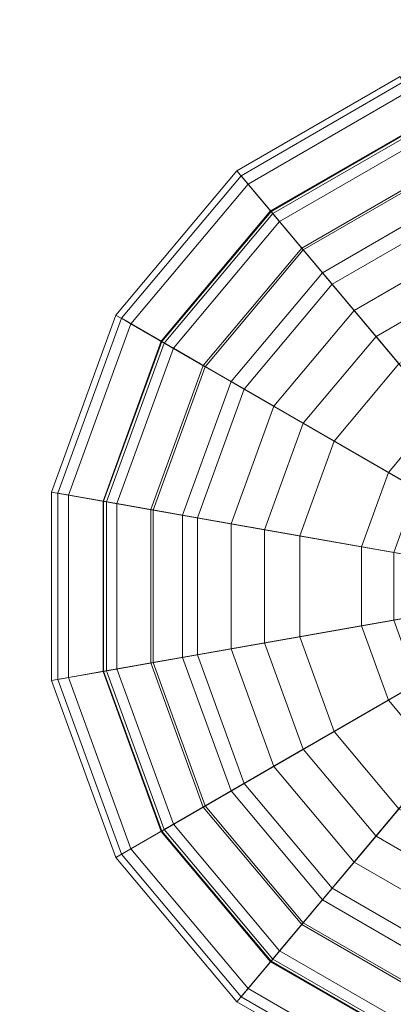
# Model space of a CAD drawing. Units: inches. Extents: x 375 to 1122, y 27 to 1069.
# Tile 128 of 155: x 720.668 to 721.601, y 901.45 to 903.908. Entities that reach past the tile are written whole.
import ezdxf

# ---------------------------------------------------------------- set-up
doc = ezdxf.new("R2010")
doc.units = ezdxf.units.IN
doc.layers.add('A-ANNO-DIMS', color=2, linetype='Continuous', lineweight=18)
doc.layers.add('Furniture', color=30, linetype='Continuous', lineweight=18)
doc.styles.get("Standard").update_dxf_attribs({"font": 'arial.ttf'})
doc.dimstyles.new('ISO-25', dxfattribs={"dimtxt": 12, "dimasz": 2.5, "dimexe": 1.5, "dimexo": 1.5, "dimtad": 1, "dimdec": 1, "dimlunit": 3, "dimtxsty": 'Standard', "dimblk": 'ARCHTICK', "dimcen": 2.5, "dimadec": 0, "dimazin": 0, "dimtfac": 1, "dimtdec": 1, "dimtmove": 0, "dimatfit": 3, "dimfxl": 1.5, "dimfxlon": 1, "dimarcsym": 0})

# ---------------------------------------------------------------- blocks, each defined once
blk = doc.blocks.new('A$C403C54AD')
for points in [[(0.863915, 0.916753, -0.042784), (0.895735, 0.928335, -0.039705), (0.895735, 0.928335, -0.039705), (0.869795, 0.906568, -0.042784)], [(0.869795, 0.906568, -0.042784), (0.895735, 0.928335, -0.039705), (0.895735, 0.928335, -0.039705), (0.878804, 0.899009, -0.042784)], [(0.878804, 0.899009, -0.042784), (0.895735, 0.928335, -0.039705), (0.895735, 0.928335, -0.039705), (0.889855, 0.894987, -0.042784)], [(0.889855, 0.894987, -0.042784), (0.895735, 0.928335, -0.039705), (0.895735, 0.928335, -0.039705), (0.901615, 0.894987, -0.042784)], [(0.921675, 0.906568, -0.042784), (0.895735, 0.928335, -0.039705), (0.895735, 0.928335, -0.039705), (0.927555, 0.916753, -0.042784)], [(0.912666, 0.899009, -0.042784), (0.895735, 0.928335, -0.039705), (0.895735, 0.928335, -0.039705), (0.921675, 0.906568, -0.042784)], [(0.901615, 0.894987, -0.042784), (0.895735, 0.928335, -0.039705), (0.895735, 0.928335, -0.039705), (0.912666, 0.899009, -0.042784)], [(0.876605, 0.921372, 0.050493), (0.886226, 0.924874, 0.043125), (0.887983, 0.92183, 0.043125), (0.88014, 0.915249, 0.050493)], [(0.911329, 0.915249, 0.050493), (0.903486, 0.92183, 0.043125), (0.905243, 0.924874, 0.043125), (0.914864, 0.921372, 0.050493)], [(0.882378, 0.923473, -0.036278), (0.866983, 0.91787, -0.039553), (0.872296, 0.908668, -0.039553), (0.884846, 0.919198, -0.036278)], [(0.906623, 0.919198, -0.036278), (0.919173, 0.908668, -0.039553), (0.924486, 0.91787, -0.039553), (0.909092, 0.923473, -0.036278)], [(0.878701, 0.922135, 0.05268), (0.872606, 0.919916, 0.062072), (0.87688, 0.912514, 0.062072), (0.881848, 0.916683, 0.05268)], [(0.888914, 0.922611, 0.046044), (0.881848, 0.916683, 0.05268), (0.886671, 0.912636, 0.05268), (0.891283, 0.920623, 0.046044)], [(0.900187, 0.920623, 0.046044), (0.904798, 0.912636, 0.05268), (0.909621, 0.916683, 0.05268), (0.902556, 0.922611, 0.046044)], [(0.909621, 0.916683, 0.05268), (0.914589, 0.912514, 0.062072), (0.918863, 0.919916, 0.062072), (0.912769, 0.922135, 0.05268)], [(0.88014, 0.915249, 0.050493), (0.887983, 0.92183, 0.043125), (0.890675, 0.919571, 0.043125), (0.885556, 0.910704, 0.050493)], [(0.905913, 0.910704, 0.050493), (0.900794, 0.919571, 0.043125), (0.903486, 0.92183, 0.043125), (0.911329, 0.915249, 0.050493)], [(0.869965, 0.918955, 0.060725), (0.876605, 0.921372, 0.050493), (0.88014, 0.915249, 0.050493), (0.874727, 0.910707, 0.060725)], [(0.916743, 0.910707, 0.060725), (0.911329, 0.915249, 0.050493), (0.914864, 0.921372, 0.050493), (0.921505, 0.918955, 0.060725)], [(0.869828, 0.918905, 0.119395), (0.874609, 0.920646, 0.129606), (0.878513, 0.913884, 0.129606), (0.874615, 0.910614, 0.119395)], [(0.874609, 0.920646, 0.129606), (0.871716, 0.919593, 0.129606), (0.876155, 0.911905, 0.129606), (0.878513, 0.913884, 0.129606)], [(0.886415, 0.920514, -0.033413), (0.884846, 0.919198, -0.036278), (0.888627, 0.916025, -0.036278), (0.889651, 0.917798, -0.033413)], [(0.891283, 0.920623, 0.046044), (0.886671, 0.912636, 0.05268), (0.892587, 0.910483, 0.05268), (0.894188, 0.919566, 0.046044)], [(0.897281, 0.919566, 0.046044), (0.898882, 0.910483, 0.05268), (0.904798, 0.912636, 0.05268), (0.900187, 0.920623, 0.046044)], [(0.901818, 0.917798, -0.033413), (0.902842, 0.916025, -0.036278), (0.906623, 0.919198, -0.036278), (0.905055, 0.920514, -0.033413)], [(0.912956, 0.913884, 0.129606), (0.915314, 0.911905, 0.129606), (0.919753, 0.919593, 0.129606), (0.91686, 0.920646, 0.129606)], [(0.916854, 0.910614, 0.119395), (0.912956, 0.913884, 0.129606), (0.91686, 0.920646, 0.129606), (0.921641, 0.918905, 0.119395)], [(0.872606, 0.919916, 0.062072), (0.867806, 0.918169, 0.079219), (0.872967, 0.90923, 0.079219), (0.87688, 0.912514, 0.062072)], [(0.914589, 0.912514, 0.062072), (0.918502, 0.90923, 0.079219), (0.923663, 0.918169, 0.079219), (0.918863, 0.919916, 0.062072)], [(0.871716, 0.919593, 0.129606), (0.867021, 0.917884, 0.1202), (0.872327, 0.908694, 0.1202), (0.876155, 0.911905, 0.129606)], [(0.884846, 0.919198, -0.036278), (0.872296, 0.908668, -0.039553), (0.880436, 0.901837, -0.039553), (0.888627, 0.916025, -0.036278)], [(0.885556, 0.910704, 0.050493), (0.890675, 0.919571, 0.043125), (0.893978, 0.91837, 0.043125), (0.8922, 0.908286, 0.050493)], [(0.894188, 0.919566, 0.046044), (0.892587, 0.910483, 0.05268), (0.898882, 0.910483, 0.05268), (0.897281, 0.919566, 0.046044)], [(0.89927, 0.908286, 0.050493), (0.897492, 0.91837, 0.043125), (0.900794, 0.919571, 0.043125), (0.905913, 0.910704, 0.050493)], [(0.902842, 0.916025, -0.036278), (0.911033, 0.901837, -0.039553), (0.919173, 0.908668, -0.039553), (0.906623, 0.919198, -0.036278)], [(0.915314, 0.911905, 0.129606), (0.919142, 0.908694, 0.1202), (0.924448, 0.917884, 0.1202), (0.919753, 0.919593, 0.129606)], [(0.864924, 0.91712, 0.078734), (0.869965, 0.918955, 0.060725), (0.874727, 0.910707, 0.060725), (0.870617, 0.907259, 0.078734)], [(0.867188, 0.917944, 0.106759), (0.869828, 0.918905, 0.119395), (0.874615, 0.910614, 0.119395), (0.872463, 0.908807, 0.106759)], [(0.920852, 0.907259, 0.078734), (0.916743, 0.910707, 0.060725), (0.921505, 0.918955, 0.060725), (0.926546, 0.91712, 0.078734)], [(0.919006, 0.908807, 0.106759), (0.916854, 0.910614, 0.119395), (0.921641, 0.918905, 0.119395), (0.924281, 0.917944, 0.106759)], [(0.866983, 0.91787, -0.039553), (0.863915, 0.916753, -0.042784), (0.869795, 0.906568, -0.042784), (0.872296, 0.908668, -0.039553)], [(0.867021, 0.917884, 0.1202), (0.864289, 0.916889, 0.106976), (0.8701, 0.906825, 0.106976), (0.872327, 0.908694, 0.1202)], [(0.867806, 0.918169, 0.079219), (0.867188, 0.917944, 0.106759), (0.872463, 0.908807, 0.106759), (0.872967, 0.90923, 0.079219)], [(0.8922, 0.908286, 0.050493), (0.893978, 0.91837, 0.043125), (0.897492, 0.91837, 0.043125), (0.89927, 0.908286, 0.050493)], [(0.918502, 0.90923, 0.079219), (0.919006, 0.908807, 0.106759), (0.924281, 0.917944, 0.106759), (0.923663, 0.918169, 0.079219)], [(0.919142, 0.908694, 0.1202), (0.921369, 0.906825, 0.106976), (0.92718, 0.916889, 0.106976), (0.924448, 0.917884, 0.1202)], [(0.919173, 0.908668, -0.039553), (0.921675, 0.906568, -0.042784), (0.927555, 0.916753, -0.042784), (0.924486, 0.91787, -0.039553)], [(0.889651, 0.917798, -0.033413), (0.888627, 0.916025, -0.036278), (0.893266, 0.914336, -0.036278), (0.893622, 0.916353, -0.033413)], [(0.897847, 0.916353, -0.033413), (0.898203, 0.914336, -0.036278), (0.902842, 0.916025, -0.036278), (0.901818, 0.917798, -0.033413)], [(0.864289, 0.916889, 0.106976), (0.864924, 0.91712, 0.078734), (0.870617, 0.907259, 0.078734), (0.8701, 0.906825, 0.106976)], [(0.881848, 0.916683, 0.05268), (0.87688, 0.912514, 0.062072), (0.883428, 0.907019, 0.062072), (0.886671, 0.912636, 0.05268)], [(0.904798, 0.912636, 0.05268), (0.908041, 0.907019, 0.062072), (0.914589, 0.912514, 0.062072), (0.909621, 0.916683, 0.05268)], [(0.921369, 0.906825, 0.106976), (0.920852, 0.907259, 0.078734), (0.926546, 0.91712, 0.078734), (0.92718, 0.916889, 0.106976)], [(0.888627, 0.916025, -0.036278), (0.880436, 0.901837, -0.039553), (0.890422, 0.898203, -0.039553), (0.893266, 0.914336, -0.036278)], [(0.893622, 0.916353, -0.033413), (0.893266, 0.914336, -0.036278), (0.898203, 0.914336, -0.036278), (0.897847, 0.916353, -0.033413)], [(0.898203, 0.914336, -0.036278), (0.901048, 0.898203, -0.039553), (0.911033, 0.901837, -0.039553), (0.902842, 0.916025, -0.036278)], [(0.874727, 0.910707, 0.060725), (0.88014, 0.915249, 0.050493), (0.885556, 0.910704, 0.050493), (0.882023, 0.904585, 0.060725)], [(0.909447, 0.904585, 0.060725), (0.905913, 0.910704, 0.050493), (0.911329, 0.915249, 0.050493), (0.916743, 0.910707, 0.060725)], [(0.893266, 0.914336, -0.036278), (0.890422, 0.898203, -0.039553), (0.901048, 0.898203, -0.039553), (0.898203, 0.914336, -0.036278)], [(0.874615, 0.910614, 0.119395), (0.878513, 0.913884, 0.129606), (0.884494, 0.908865, 0.129606), (0.88195, 0.904459, 0.119395)], [(0.878513, 0.913884, 0.129606), (0.876155, 0.911905, 0.129606), (0.882955, 0.906199, 0.129606), (0.884494, 0.908865, 0.129606)], [(0.906975, 0.908865, 0.129606), (0.908514, 0.906199, 0.129606), (0.915314, 0.911905, 0.129606), (0.912956, 0.913884, 0.129606)], [(0.909519, 0.904459, 0.119395), (0.906975, 0.908865, 0.129606), (0.912956, 0.913884, 0.129606), (0.916854, 0.910614, 0.119395)], [(0.87688, 0.912514, 0.062072), (0.872967, 0.90923, 0.079219), (0.880874, 0.902596, 0.079219), (0.883428, 0.907019, 0.062072)], [(0.886671, 0.912636, 0.05268), (0.883428, 0.907019, 0.062072), (0.891461, 0.904095, 0.062072), (0.892587, 0.910483, 0.05268)], [(0.898882, 0.910483, 0.05268), (0.900009, 0.904095, 0.062072), (0.908041, 0.907019, 0.062072), (0.904798, 0.912636, 0.05268)], [(0.908041, 0.907019, 0.062072), (0.910595, 0.902596, 0.079219), (0.918502, 0.90923, 0.079219), (0.914589, 0.912514, 0.062072)], [(0.876155, 0.911905, 0.129606), (0.872327, 0.908694, 0.1202), (0.880457, 0.901872, 0.1202), (0.882955, 0.906199, 0.129606)], [(0.908514, 0.906199, 0.129606), (0.911013, 0.901872, 0.1202), (0.919142, 0.908694, 0.1202), (0.915314, 0.911905, 0.129606)], [(0.870617, 0.907259, 0.078734), (0.874727, 0.910707, 0.060725), (0.882023, 0.904585, 0.060725), (0.87934, 0.899939, 0.078734)], [(0.872463, 0.908807, 0.106759), (0.874615, 0.910614, 0.119395), (0.88195, 0.904459, 0.119395), (0.880545, 0.902026, 0.106759)], [(0.882023, 0.904585, 0.060725), (0.885556, 0.910704, 0.050493), (0.8922, 0.908286, 0.050493), (0.890973, 0.901327, 0.060725)], [(0.892587, 0.910483, 0.05268), (0.891461, 0.904095, 0.062072), (0.900009, 0.904095, 0.062072), (0.898882, 0.910483, 0.05268)], [(0.900497, 0.901327, 0.060725), (0.89927, 0.908286, 0.050493), (0.905913, 0.910704, 0.050493), (0.909447, 0.904585, 0.060725)], [(0.912129, 0.899939, 0.078734), (0.909447, 0.904585, 0.060725), (0.916743, 0.910707, 0.060725), (0.920852, 0.907259, 0.078734)], [(0.910924, 0.902026, 0.106759), (0.909519, 0.904459, 0.119395), (0.916854, 0.910614, 0.119395), (0.919006, 0.908807, 0.106759)], [(0.872967, 0.90923, 0.079219), (0.872463, 0.908807, 0.106759), (0.880545, 0.902026, 0.106759), (0.880874, 0.902596, 0.079219)], [(0.910595, 0.902596, 0.079219), (0.910924, 0.902026, 0.106759), (0.919006, 0.908807, 0.106759), (0.918502, 0.90923, 0.079219)], [(0.872296, 0.908668, -0.039553), (0.869795, 0.906568, -0.042784), (0.878804, 0.899009, -0.042784), (0.880436, 0.901837, -0.039553)], [(0.872327, 0.908694, 0.1202), (0.8701, 0.906825, 0.106976), (0.879003, 0.899355, 0.106976), (0.880457, 0.901872, 0.1202)], [(0.88195, 0.904459, 0.119395), (0.884494, 0.908865, 0.129606), (0.891831, 0.906195, 0.129606), (0.890947, 0.901184, 0.119395)], [(0.884494, 0.908865, 0.129606), (0.882955, 0.906199, 0.129606), (0.891296, 0.903163, 0.129606), (0.891831, 0.906195, 0.129606)], [(0.899638, 0.906195, 0.129606), (0.900173, 0.903163, 0.129606), (0.908514, 0.906199, 0.129606), (0.906975, 0.908865, 0.129606)], [(0.900522, 0.901184, 0.119395), (0.899638, 0.906195, 0.129606), (0.906975, 0.908865, 0.129606), (0.909519, 0.904459, 0.119395)], [(0.911013, 0.901872, 0.1202), (0.912466, 0.899355, 0.106976), (0.921369, 0.906825, 0.106976), (0.919142, 0.908694, 0.1202)], [(0.911033, 0.901837, -0.039553), (0.912666, 0.899009, -0.042784), (0.921675, 0.906568, -0.042784), (0.919173, 0.908668, -0.039553)], [(0.890973, 0.901327, 0.060725), (0.8922, 0.908286, 0.050493), (0.89927, 0.908286, 0.050493), (0.900497, 0.901327, 0.060725)], [(0.8701, 0.906825, 0.106976), (0.870617, 0.907259, 0.078734), (0.87934, 0.899939, 0.078734), (0.879003, 0.899355, 0.106976)], [(0.883428, 0.907019, 0.062072), (0.880874, 0.902596, 0.079219), (0.890574, 0.899065, 0.079219), (0.891461, 0.904095, 0.062072)], [(0.900009, 0.904095, 0.062072), (0.900896, 0.899065, 0.079219), (0.910595, 0.902596, 0.079219), (0.908041, 0.907019, 0.062072)], [(0.912466, 0.899355, 0.106976), (0.912129, 0.899939, 0.078734), (0.920852, 0.907259, 0.078734), (0.921369, 0.906825, 0.106976)], [(0.882955, 0.906199, 0.129606), (0.880457, 0.901872, 0.1202), (0.890429, 0.898243, 0.1202), (0.891296, 0.903163, 0.129606)], [(0.890947, 0.901184, 0.119395), (0.891831, 0.906195, 0.129606), (0.899638, 0.906195, 0.129606), (0.900522, 0.901184, 0.119395)], [(0.891831, 0.906195, 0.129606), (0.891296, 0.903163, 0.129606), (0.900173, 0.903163, 0.129606), (0.899638, 0.906195, 0.129606)], [(0.900173, 0.903163, 0.129606), (0.901041, 0.898243, 0.1202), (0.911013, 0.901872, 0.1202), (0.908514, 0.906199, 0.129606)], [(0.87934, 0.899939, 0.078734), (0.882023, 0.904585, 0.060725), (0.890973, 0.901327, 0.060725), (0.890041, 0.896044, 0.078734)], [(0.880545, 0.902026, 0.106759), (0.88195, 0.904459, 0.119395), (0.890947, 0.901184, 0.119395), (0.890459, 0.898417, 0.106759)], [(0.901428, 0.896044, 0.078734), (0.900497, 0.901327, 0.060725), (0.909447, 0.904585, 0.060725), (0.912129, 0.899939, 0.078734)], [(0.90101, 0.898417, 0.106759), (0.900522, 0.901184, 0.119395), (0.909519, 0.904459, 0.119395), (0.910924, 0.902026, 0.106759)], [(0.891461, 0.904095, 0.062072), (0.890574, 0.899065, 0.079219), (0.900896, 0.899065, 0.079219), (0.900009, 0.904095, 0.062072)], [(0.891296, 0.903163, 0.129606), (0.890429, 0.898243, 0.1202), (0.901041, 0.898243, 0.1202), (0.900173, 0.903163, 0.129606)], [(0.880874, 0.902596, 0.079219), (0.880545, 0.902026, 0.106759), (0.890459, 0.898417, 0.106759), (0.890574, 0.899065, 0.079219)], [(0.900896, 0.899065, 0.079219), (0.90101, 0.898417, 0.106759), (0.910924, 0.902026, 0.106759), (0.910595, 0.902596, 0.079219)], [(0.880436, 0.901837, -0.039553), (0.878804, 0.899009, -0.042784), (0.889855, 0.894987, -0.042784), (0.890422, 0.898203, -0.039553)], [(0.880457, 0.901872, 0.1202), (0.879003, 0.899355, 0.106976), (0.889924, 0.89538, 0.106976), (0.890429, 0.898243, 0.1202)], [(0.901041, 0.898243, 0.1202), (0.901545, 0.89538, 0.106976), (0.912466, 0.899355, 0.106976), (0.911013, 0.901872, 0.1202)], [(0.901048, 0.898203, -0.039553), (0.901615, 0.894987, -0.042784), (0.912666, 0.899009, -0.042784), (0.911033, 0.901837, -0.039553)], [(0.890041, 0.896044, 0.078734), (0.890973, 0.901327, 0.060725), (0.900497, 0.901327, 0.060725), (0.901428, 0.896044, 0.078734)], [(0.890459, 0.898417, 0.106759), (0.890947, 0.901184, 0.119395), (0.900522, 0.901184, 0.119395), (0.90101, 0.898417, 0.106759)], [(0.879003, 0.899355, 0.106976), (0.87934, 0.899939, 0.078734), (0.890041, 0.896044, 0.078734), (0.889924, 0.89538, 0.106976)], [(0.901545, 0.89538, 0.106976), (0.901428, 0.896044, 0.078734), (0.912129, 0.899939, 0.078734), (0.912466, 0.899355, 0.106976)], [(0.890574, 0.899065, 0.079219), (0.890459, 0.898417, 0.106759), (0.90101, 0.898417, 0.106759), (0.900896, 0.899065, 0.079219)], [(0.890422, 0.898203, -0.039553), (0.889855, 0.894987, -0.042784), (0.901615, 0.894987, -0.042784), (0.901048, 0.898203, -0.039553)], [(0.890429, 0.898243, 0.1202), (0.889924, 0.89538, 0.106976), (0.901545, 0.89538, 0.106976), (0.901041, 0.898243, 0.1202)], [(0.889924, 0.89538, 0.106976), (0.890041, 0.896044, 0.078734), (0.901428, 0.896044, 0.078734), (0.901545, 0.89538, 0.106976)]]:
    blk.add_3dface(points)
blk = doc.blocks.new('_ArchTick')
at = {"color": 0, "linetype": 'ByBlock', "const_width": 0.15}
blk.add_lwpolyline([(-0.5, -0.5), (0.5, 0.5)], dxfattribs=at)
blk = doc.blocks.new('*D73')
at = {"layer": 'A-ANNO-DIMS', "color": 0, "lineweight": -2, "transparency": 16777216}
for p, q in [((686.7573, 932.4277), (686.7573, 929.4277)), ((770.7573, 932.4277), (770.7573, 929.4277)), ((686.7573, 930.9277), (770.7573, 930.9277)), ((770.7573, 930.9277), (987.6096, 930.9277))]:
    blk.add_line(p, q, dxfattribs=at)
at = {"layer": 'Defpoints', "color": 0, "transparency": 16777216}
for p in [(686.7573, 943.5277), (770.7573, 943.5277), (770.7573, 930.9277)]:
    blk.add_point(p, dxfattribs=at)
at = {"layer": 'A-ANNO-DIMS', "color": 0, "lineweight": -2, "transparency": 16777216, "xscale": 2.5, "yscale": 2.5, "zscale": 2.5, "rotation": 180}
blk.add_blockref('_ArchTick', (686.7573, 930.9277), dxfattribs=at)
at = {"layer": 'A-ANNO-DIMS', "color": 0, "lineweight": -2, "transparency": 16777216, "xscale": 2.5, "yscale": 2.5, "zscale": 2.5}
blk.add_blockref('_ArchTick', (770.7573, 930.9277), dxfattribs=at)
at = {"layer": 'A-ANNO-DIMS', "color": 0, "transparency": 16777216, "insert": (880.4335, 937.7573), "char_height": 12, "attachment_point": 5}
blk.add_mtext('2-PANEL SLIDER 7\'-0" TYP.', dxfattribs=at)

msp = doc.modelspace()

# ---------------------------------------------------------------- block references
at = {"layer": 'Furniture', "xscale": 39.9918517141215, "yscale": 39.9918517141215, "zscale": 39.9918517141215, "rotation": 270}
msp.add_blockref('A$C403C54AD', (684.9549, 938.3156, 0.024), dxfattribs=at)

# ---------------------------------------------------------------- dimensions: what is measured, and where the dimension line sits
at = {"layer": 'A-ANNO-DIMS'}
dim = msp.add_linear_dim(base=(770.7573, 930.9277), p1=(686.7573, 943.5277), p2=(770.7573, 943.5277), text='2-PANEL SLIDER <> TYP.', dimstyle='ISO-25', override={"dimdec": 1, "dimlfac": 1, "dimrnd": 0, "dimzin": 1, "dimdsep": 46, "dimlunit": 4, "dimfrac": 2}, dxfattribs=at)
dim.commit()
dim.dimension.update_dxf_attribs({"geometry": '*D73', "text_midpoint": (880.4335, 937.7573)})

doc.saveas('drawing.dxf')
